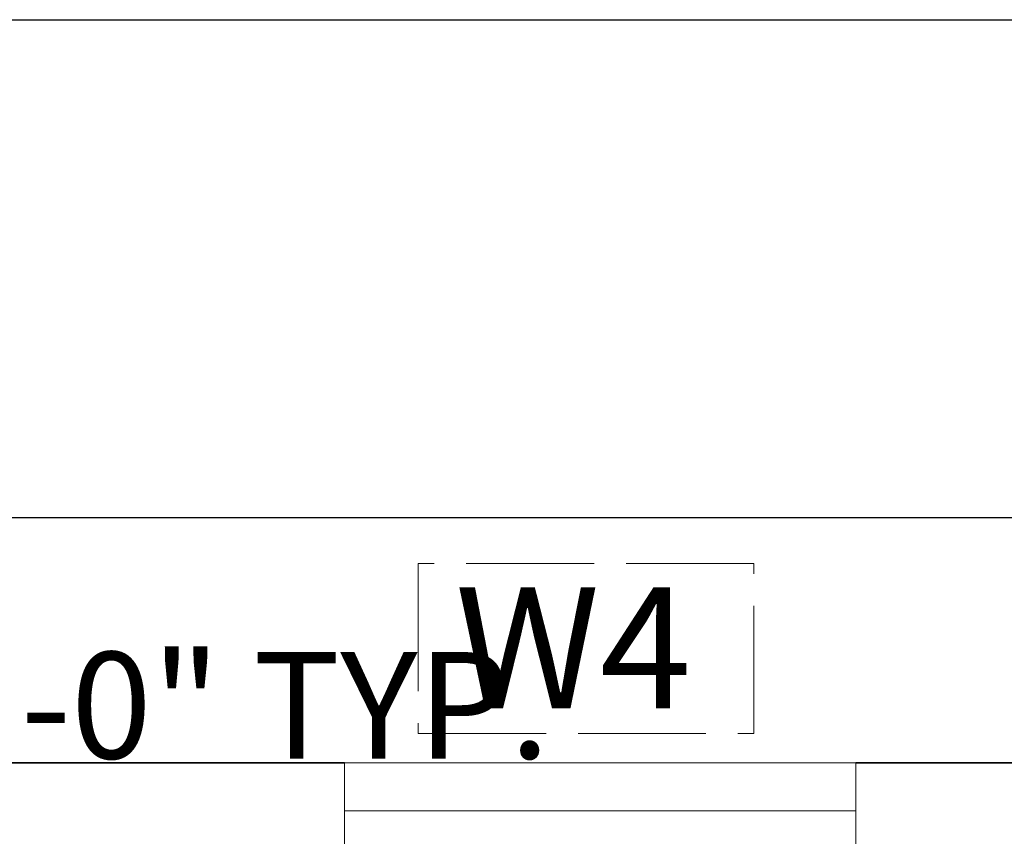
# Model space of a CAD drawing. Units: inches. Extents: x -269 to 4574, y -694 to 313.
# Tile 14 of 19: x 302 to 395, y 11 to 88. Entities that reach past the tile are written whole.
import ezdxf

# ---------------------------------------------------------------- set-up
doc = ezdxf.new("R2010")
doc.units = ezdxf.units.IN
doc.header["$MEASUREMENT"] = 0
doc.linetypes.add('ACAD_ISO02W100', pattern=[15, 12, -3])
for name, color, linetype, lineweight in [('A-ANNO-FRAM', 7, 'ACAD_ISO02W100', 13), ('A-ANNO-IDEN', 6, 'Continuous', 18), ('C-PROP', 7, 'Continuous', 25), ('DIMENSION', 5, 'Continuous', 18), ('WALL', 1, 'Continuous', 35), ('WINDOWS', 2, 'Continuous', 18)]:
    doc.layers.add(name, color=color, linetype=linetype, lineweight=lineweight)
doc.dimstyles.get("Standard").update_dxf_attribs({"dimtxt": 10, "dimasz": 0.18, "dimexe": 0.18, "dimexo": 0.0625, "dimgap": 0.09, "dimtad": 0, "dimdec": 1, "dimzin": 0, "dimdsep": 46, "dimlunit": 3, "dimtxsty": 'Standard', "dimcen": 0.09, "dimclrt": 7, "dimadec": 0, "dimazin": 0, "dimtfac": 1, "dimtdec": 1, "dimtofl": 0, "dimtmove": 0, "dimatfit": 3, "dimfxl": 1, "dimtolj": 1, "dimtzin": 0, "dimarcsym": 0})

# ---------------------------------------------------------------- blocks, each defined once
blk = doc.blocks.new('*D1')
at = {"layer": 'Defpoints', "color": 0, "lineweight": 0, "transparency": 16777216}
for p in [(451.137, 41.262), (7.137, 18.268), (451.137, 18.268)]:
    blk.add_point(p, dxfattribs=at)
at = {"layer": 'DIMENSION', "color": 0, "lineweight": -2, "transparency": 16777216}
for p, q in [((7.137, 18.331), (7.137, 41.442)), ((7.317, 41.262), (219.047, 41.262)), ((450.957, 41.262), (239.227, 41.262)), ((451.137, 18.331), (451.137, 41.442))]:
    blk.add_line(p, q, dxfattribs=at)
at = {"layer": 'DIMENSION', "color": 0, "lineweight": 0, "transparency": 16777216}
for points in [[(7.317, 41.292), (7.317, 41.232), (7.137, 41.262)], [(450.957, 41.292), (450.957, 41.232), (451.137, 41.262)]]:
    blk.add_solid(points, dxfattribs=at)
at = {"layer": 'DIMENSION', "color": 0, "transparency": 16777216, "insert": (229.137, 41.262), "char_height": 10, "attachment_point": 5}
blk.add_mtext("\\A1;37'", dxfattribs=at)
blk = doc.blocks.new('GLAZ-48IN')
blk.add_line((4.5, 0), (4.5, 48))
blk.add_lwpolyline([(0, 48), (9, 48), (9, 0), (0, 0)], close=True)
blk = doc.blocks.new('*D55')
at = {"layer": 'Defpoints', "color": 0, "lineweight": 0, "transparency": 16777216}
for p in [(217.137, 23.668), (181.137, 18.268), (217.137, 18.268)]:
    blk.add_point(p, dxfattribs=at)
at = {"layer": 'DIMENSION', "color": 0, "lineweight": -2, "transparency": 16777216}
for p, q in [((181.137, 18.331), (181.137, 23.848)), ((181.317, 23.668), (216.957, 23.668)), ((217.137, 18.331), (217.137, 23.848)), ((217.137, 23.668), (217.317, 23.668))]:
    blk.add_line(p, q, dxfattribs=at)
at = {"layer": 'DIMENSION', "color": 0, "lineweight": 0, "transparency": 16777216}
for points in [[(181.317, 23.698), (181.317, 23.638), (181.137, 23.668)], [(216.957, 23.698), (216.957, 23.638), (217.137, 23.668)]]:
    blk.add_solid(points, dxfattribs=at)
at = {"layer": 'DIMENSION', "color": 7, "transparency": 16777216, "insert": (291.217, 23.668), "char_height": 10, "attachment_point": 5}
blk.add_mtext('\\A1;WINDOW 3\'-0" TYP.', dxfattribs=at)

msp = doc.modelspace()

# ---------------------------------------------------------------- linework, layer by layer
at = {"layer": 'A-ANNO-FRAM'}
msp.add_lwpolyline([(371.072, 36.977), (339.573, 36.977), (339.573, 21.01), (371.072, 21.01)], close=True, dxfattribs=at)
at = {"layer": 'C-PROP'}
msp.add_line((-37.705, 88), (478.295, 88), dxfattribs=at)
at = {"layer": 'WALL'}
for p, q in [((217.137, 18.268), (332.637, 18.268)), ((380.637, 18.268), (451.137, 18.268))]:
    msp.add_line(p, q, dxfattribs=at)

# ---------------------------------------------------------------- block references
at = {"layer": 'WINDOWS', "extrusion": (0, 0, -1), "zscale": -1, "rotation": 269.9999999999999}
msp.add_blockref('GLAZ-48IN', (-380.637, 18.268), dxfattribs=at)

# ---------------------------------------------------------------- texts
at = {"layer": 'A-ANNO-IDEN'}
msp.add_text('W4', height=11.343, dxfattribs=at).set_placement((343.027, 23.385))

# ---------------------------------------------------------------- dimensions: what is measured, and where the dimension line sits
at = {"layer": 'DIMENSION'}
dim = msp.add_linear_dim(base=(451.137, 41.262), p1=(7.137, 18.268), p2=(451.137, 18.268), dimstyle='Standard', override={"dimclrd": 0, "dimclre": 0, "dimclrt": 0}, dxfattribs=at)
dim.commit()
dim.dimension.update_dxf_attribs({"geometry": '*D1', "text_midpoint": (229.137, 41.262)})
dim = msp.add_linear_dim(base=(217.137, 23.668), p1=(181.137, 18.268), p2=(217.137, 18.268), text='WINDOW <> TYP.', dimstyle='Standard', override={"dimdec": 1, "dimlfac": 1, "dimrnd": 0, "dimzin": 1, "dimdsep": 46, "dimlunit": 4, "dimfrac": 2}, dxfattribs=at)
dim.commit()
dim.dimension.update_dxf_attribs({"geometry": '*D55', "text_midpoint": (291.217, 23.668)})

doc.saveas('drawing.dxf')
